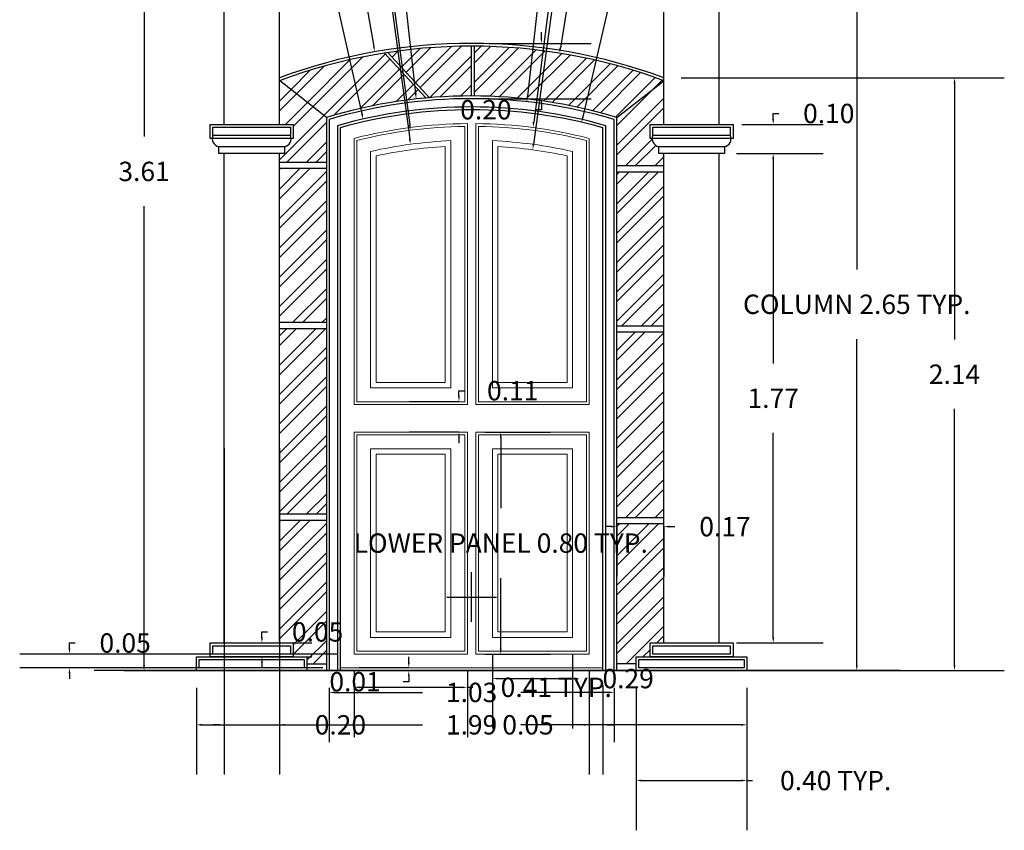
# Model space of a CAD drawing. Units: metres. Extents: x 10.71 to 14.27, y 9.22 to 13.79.
# Tile 1 of 2: x 10.71 to 14.27, y 9.22 to 12.15. Entities that reach past the tile are written whole.
import ezdxf

# ---------------------------------------------------------------- set-up
doc = ezdxf.new("R2010")
doc.units = ezdxf.units.M
doc.header["$MEASUREMENT"] = 0
for name, color, linetype, lineweight in [('A-ANNO-DIMS', 2, 'Continuous', 18), ('A-COLS', 7, 'Continuous', 30), ('A-DOOR', 4, 'Continuous', 18), ('A-DOOR-FRAM', 4, 'Continuous', 25), ('A-ELEV-GRND', 7, 'Continuous', 35), ('A-WALL', 7, 'Continuous', 25), ('A-WALL-PATT', 252, 'Continuous', 13)]:
    doc.layers.add(name, color=color, linetype=linetype, lineweight=lineweight)
doc.styles.get("Standard").update_dxf_attribs({"font": 'arial.ttf'})
doc.dimstyles.get("Standard").update_dxf_attribs({"dimtxt": 0.07, "dimasz": 0.02, "dimexe": 0.18, "dimexo": 0.0625, "dimgap": 0.09, "dimtad": 0, "dimtih": 1, "dimtoh": 1, "dimzin": 0, "dimdsep": 46, "dimtxsty": 'Standard', "dimcen": 0.09, "dimadec": 0, "dimazin": 0, "dimtfac": 1, "dimtofl": 0, "dimtmove": 0, "dimatfit": 3, "dimfxl": 1, "dimfxlon": 1, "dimtolj": 1, "dimtzin": 0, "dimarcsym": 0})

# ---------------------------------------------------------------- blocks, each defined once
blk = doc.blocks.new('*D1')
at = {"layer": 'A-ANNO-DIMS', "color": 0, "lineweight": -2, "transparency": 16777216}
for p, q in [((12.8472, 10.321), (12.8272, 10.321)), ((12.8672, 10.321), (12.8672, 10.141)), ((13.0372, 10.321), (13.0372, 10.141)), ((13.0572, 10.321), (13.0772, 10.321))]:
    blk.add_line(p, q, dxfattribs=at)
at = {"layer": 'A-ANNO-DIMS', "color": 0, "transparency": 16777216}
for points in [[(12.8472, 10.3244), (12.8472, 10.3177), (12.8672, 10.321)], [(13.0572, 10.3244), (13.0572, 10.3177), (13.0372, 10.321)]]:
    blk.add_solid(points, dxfattribs=at)
at = {"layer": 'Defpoints', "color": 0, "transparency": 16777216}
for p in [(12.8672, 10.332), (13.0372, 10.332), (13.0372, 10.321)]:
    blk.add_point(p, dxfattribs=at)
at = {"layer": 'A-ANNO-DIMS', "color": 0, "transparency": 16777216, "insert": (13.2581, 10.321), "char_height": 0.07, "attachment_point": 5}
blk.add_mtext('\\A1;0.17', dxfattribs=at)
blk = doc.blocks.new('*D2')
at = {"layer": 'A-ANNO-DIMS', "color": 0, "lineweight": -2, "transparency": 16777216}
for p, q in [((13.4325, 11.795), (13.4325, 11.815)), ((13.4325, 11.815), (13.4525, 11.815)), ((13.3185, 11.775), (13.6125, 11.775)), ((13.3185, 11.6703), (13.6125, 11.6703)), ((13.4325, 11.6503), (13.4325, 11.6303))]:
    blk.add_line(p, q, dxfattribs=at)
at = {"layer": 'A-ANNO-DIMS', "color": 0, "transparency": 16777216}
for points in [[(13.4291, 11.795), (13.4358, 11.795), (13.4325, 11.775)], [(13.4291, 11.6503), (13.4358, 11.6503), (13.4325, 11.6703)]]:
    blk.add_solid(points, dxfattribs=at)
at = {"layer": 'Defpoints', "color": 0, "transparency": 16777216}
for p in [(13.256, 11.775), (13.4325, 11.775), (13.256, 11.6703)]:
    blk.add_point(p, dxfattribs=at)
at = {"layer": 'A-ANNO-DIMS', "color": 0, "transparency": 16777216, "insert": (13.6333, 11.815), "char_height": 0.07, "attachment_point": 5}
blk.add_mtext('\\A1;0.10', dxfattribs=at)
blk = doc.blocks.new('*D3')
at = {"layer": 'A-ANNO-DIMS', "color": 0, "lineweight": -2, "transparency": 16777216}
for p, q in [((13.2997, 11.6703), (13.6125, 11.6703)), ((13.4325, 11.6503), (13.4325, 10.9104)), ((13.4325, 9.9203), (13.4325, 10.6601)), ((13.2997, 9.9003), (13.6125, 9.9003))]:
    blk.add_line(p, q, dxfattribs=at)
at = {"layer": 'A-ANNO-DIMS', "color": 0, "transparency": 16777216}
for points in [[(13.4291, 11.6503), (13.4358, 11.6503), (13.4325, 11.6703)], [(13.4291, 9.9203), (13.4358, 9.9203), (13.4325, 9.9003)]]:
    blk.add_solid(points, dxfattribs=at)
at = {"layer": 'Defpoints', "color": 0, "transparency": 16777216}
for p in [(13.2372, 11.6703), (13.4325, 11.6703), (13.2372, 9.9003)]:
    blk.add_point(p, dxfattribs=at)
at = {"layer": 'A-ANNO-DIMS', "color": 0, "transparency": 16777216, "insert": (13.4325, 10.7853), "char_height": 0.07, "attachment_point": 5}
blk.add_mtext('\\A1;1.77', dxfattribs=at)
blk = doc.blocks.new('*D4')
at = {"layer": 'A-ANNO-DIMS', "color": 0, "lineweight": -2, "transparency": 16777216}
for p, q in [((12.1582, 13.4108), (10.9782, 13.4108)), ((11.1582, 13.3908), (11.1582, 11.7313)), ((11.1582, 9.8203), (11.1582, 11.4798)), ((11.1582, 9.8003), (10.9782, 9.8003))]:
    blk.add_line(p, q, dxfattribs=at)
at = {"layer": 'A-ANNO-DIMS', "color": 0, "transparency": 16777216}
for points in [[(11.1548, 13.3908), (11.1615, 13.3908), (11.1582, 13.4108)], [(11.1548, 9.8203), (11.1615, 9.8203), (11.1582, 9.8003)]]:
    blk.add_solid(points, dxfattribs=at)
at = {"layer": 'Defpoints', "color": 0, "transparency": 16777216}
for p in [(11.1582, 13.4108), (12.3422, 13.4108), (11.1842, 9.8003)]:
    blk.add_point(p, dxfattribs=at)
at = {"layer": 'A-ANNO-DIMS', "color": 0, "transparency": 16777216, "insert": (11.1582, 11.6055), "char_height": 0.07, "attachment_point": 5}
blk.add_mtext('\\A1;3.61', dxfattribs=at)
blk = doc.blocks.new('*D6')
at = {"layer": 'A-ANNO-DIMS', "color": 0, "lineweight": -2, "transparency": 16777216}
for p, q in [((12.5946, 12.0885), (12.5946, 12.1085)), ((12.4047, 12.0685), (12.7746, 12.0685)), ((12.4047, 11.8685), (12.7746, 11.8685)), ((12.5946, 11.8285), (12.5746, 11.8285)), ((12.5946, 11.8485), (12.5946, 11.8285))]:
    blk.add_line(p, q, dxfattribs=at)
at = {"layer": 'A-ANNO-DIMS', "color": 0, "transparency": 16777216}
for points in [[(12.5912, 12.0885), (12.5979, 12.0885), (12.5946, 12.0685)], [(12.5912, 11.8485), (12.5979, 11.8485), (12.5946, 11.8685)]]:
    blk.add_solid(points, dxfattribs=at)
at = {"layer": 'Defpoints', "color": 0, "transparency": 16777216}
for p in [(12.3422, 12.0685), (12.3422, 11.8685), (12.5946, 11.8685)]:
    blk.add_point(p, dxfattribs=at)
at = {"layer": 'A-ANNO-DIMS', "color": 0, "transparency": 16777216, "insert": (12.3938, 11.8285), "char_height": 0.07, "attachment_point": 5}
blk.add_mtext('\\A1;0.20', dxfattribs=at)
blk = doc.blocks.new('*D7')
at = {"layer": 'A-ANNO-DIMS', "color": 0, "lineweight": -2, "transparency": 16777216}
for p, q in [((12.2966, 10.7926), (12.2966, 10.8126)), ((12.2966, 10.8126), (12.3166, 10.8126)), ((12.2966, 10.7726), (12.1166, 10.7726)), ((12.2966, 10.6626), (12.1166, 10.6626)), ((12.2966, 10.6426), (12.2966, 10.6226))]:
    blk.add_line(p, q, dxfattribs=at)
at = {"layer": 'A-ANNO-DIMS', "color": 0, "transparency": 16777216}
for points in [[(12.2933, 10.7926), (12.3, 10.7926), (12.2966, 10.7726)], [(12.2933, 10.6426), (12.3, 10.6426), (12.2966, 10.6626)]]:
    blk.add_solid(points, dxfattribs=at)
at = {"layer": 'Defpoints', "color": 0, "transparency": 16777216}
for p in [(12.2966, 10.7726), (12.3172, 10.7726), (12.3272, 10.6626)]:
    blk.add_point(p, dxfattribs=at)
at = {"layer": 'A-ANNO-DIMS', "color": 0, "transparency": 16777216, "insert": (12.4908, 10.8126), "char_height": 0.07, "attachment_point": 5}
blk.add_mtext('\\A1;0.11', dxfattribs=at)
blk = doc.blocks.new('*D8')
at = {"layer": 'A-ANNO-DIMS', "color": 0, "lineweight": -2, "transparency": 16777216}
for p, q in [((11.5843, 9.9203), (11.5843, 9.9403)), ((11.5843, 9.9403), (11.6043, 9.9403)), ((11.5843, 9.9003), (11.7643, 9.9003)), ((11.5843, 9.8503), (11.7643, 9.8503)), ((11.5843, 9.8303), (11.5843, 9.8103))]:
    blk.add_line(p, q, dxfattribs=at)
at = {"layer": 'A-ANNO-DIMS', "color": 0, "transparency": 16777216}
for points in [[(11.581, 9.9203), (11.5877, 9.9203), (11.5843, 9.9003)], [(11.581, 9.8303), (11.5877, 9.8303), (11.5843, 9.8503)]]:
    blk.add_solid(points, dxfattribs=at)
at = {"layer": 'Defpoints', "color": 0, "transparency": 16777216}
for p in [(11.5582, 9.9003), (11.5843, 9.9003), (11.5582, 9.8503)]:
    blk.add_point(p, dxfattribs=at)
at = {"layer": 'A-ANNO-DIMS', "color": 0, "transparency": 16777216, "insert": (11.7855, 9.9403), "char_height": 0.07, "attachment_point": 5}
blk.add_mtext('\\A1;0.05', dxfattribs=at)
blk = doc.blocks.new('*D10')
at = {"layer": 'A-ANNO-DIMS', "color": 0, "lineweight": -2, "transparency": 16777216}
for p, q in [((11.8272, 9.7378), (11.8272, 9.5415)), ((11.8472, 9.7215), (12.1646, 9.7215)), ((12.8372, 9.7215), (12.5198, 9.7215)), ((12.8572, 9.7378), (12.8572, 9.5415))]:
    blk.add_line(p, q, dxfattribs=at)
at = {"layer": 'A-ANNO-DIMS', "color": 0, "transparency": 16777216}
for points in [[(11.8472, 9.7248), (11.8472, 9.7182), (11.8272, 9.7215)], [(12.8372, 9.7248), (12.8372, 9.7182), (12.8572, 9.7215)]]:
    blk.add_solid(points, dxfattribs=at)
at = {"layer": 'Defpoints', "color": 0, "transparency": 16777216}
for p in [(11.8272, 9.8003), (12.8572, 9.8003), (12.8572, 9.7215)]:
    blk.add_point(p, dxfattribs=at)
at = {"layer": 'A-ANNO-DIMS', "color": 0, "transparency": 16777216, "insert": (12.3422, 9.7215), "char_height": 0.07, "attachment_point": 5}
blk.add_mtext('\\A1;1.03', dxfattribs=at)
blk = doc.blocks.new('*D11')
at = {"layer": 'A-ANNO-DIMS', "color": 0, "lineweight": -2, "transparency": 16777216}
for p, q in [((12.1152, 9.8302), (12.1152, 9.8502)), ((12.1152, 9.8102), (11.9352, 9.8102)), ((12.1152, 9.8003), (11.9352, 9.8003)), ((12.1152, 9.7603), (12.0952, 9.7603)), ((12.1152, 9.7803), (12.1152, 9.7603))]:
    blk.add_line(p, q, dxfattribs=at)
at = {"layer": 'A-ANNO-DIMS', "color": 0, "transparency": 16777216}
for points in [[(12.1118, 9.8302), (12.1185, 9.8302), (12.1152, 9.8102)], [(12.1118, 9.7803), (12.1185, 9.7803), (12.1152, 9.8003)]]:
    blk.add_solid(points, dxfattribs=at)
at = {"layer": 'Defpoints', "color": 0, "transparency": 16777216}
for p in [(12.1152, 9.8003), (12.1372, 9.8102), (12.1372, 9.8003)]:
    blk.add_point(p, dxfattribs=at)
at = {"layer": 'A-ANNO-DIMS', "color": 0, "transparency": 16777216, "insert": (11.921, 9.7603), "char_height": 0.07, "attachment_point": 5}
blk.add_mtext('\\A1;0.01', dxfattribs=at)
blk = doc.blocks.new('*D12')
at = {"layer": 'A-ANNO-DIMS', "color": 0, "lineweight": -2, "transparency": 16777216}
for p, q in [((12.4172, 9.8577), (12.4172, 9.5915)), ((12.7072, 9.8577), (12.7072, 9.5915)), ((12.4372, 9.7715), (12.6872, 9.7715)), ((12.7072, 9.7715), (12.7272, 9.7715))]:
    blk.add_line(p, q, dxfattribs=at)
at = {"layer": 'A-ANNO-DIMS', "color": 0, "transparency": 16777216}
for points in [[(12.4372, 9.7748), (12.4372, 9.7682), (12.4172, 9.7715)], [(12.6872, 9.7748), (12.6872, 9.7682), (12.7072, 9.7715)]]:
    blk.add_solid(points, dxfattribs=at)
at = {"layer": 'Defpoints', "color": 0, "transparency": 16777216}
for p in [(12.4172, 9.9202), (12.7072, 9.9202), (12.7072, 9.7715)]:
    blk.add_point(p, dxfattribs=at)
at = {"layer": 'A-ANNO-DIMS', "color": 0, "transparency": 16777216, "insert": (12.9082, 9.7715), "char_height": 0.07, "attachment_point": 5}
blk.add_mtext('\\A1;0.29', dxfattribs=at)
blk = doc.blocks.new('COL-ENTRANCE-CLASSICAL')
for p, q in [((0.1002, 1.975), (0.1002, 2.545)), ((0.3002, 1.975), (0.3002, 2.545)), ((0.1002, 0.1003), (0.1002, 1.8703)), ((0.3002, 0.1003), (0.3002, 1.8703)), ((0.1002, 0.1003), (0.3002, 0.1003))]:
    blk.add_line(p, q)
for points in [[(0.0502, 2.6498), (0.3502, 2.6498), (0.3502, 2.5998), (0.0502, 2.5998)], [(0.0602, 2.6398), (0.3402, 2.6398), (0.3402, 2.6098), (0.0602, 2.6098)], [(0.0816, 2.5705), (0.319, 2.5705), (0.319, 2.545), (0.0816, 2.545)], [(0.0502, 1.975), (0.3502, 1.975), (0.3502, 1.925), (0.0502, 1.925)], [(0.0602, 1.965), (0.3402, 1.965), (0.3402, 1.935), (0.0602, 1.935)], [(0.0816, 1.8957), (0.319, 1.8957), (0.319, 1.8703), (0.0816, 1.8703)], [(0.0502, 0.1003), (0.3502, 0.1003), (0.3502, 0.0503), (0.0502, 0.0503)], [(0.0602, 0.0903), (0.3402, 0.0903), (0.3402, 0.0603), (0.0602, 0.0603)], [(0.0002, 0.0503), (0.4002, 0.0503), (0.4002, 0.0003), (0.0002, 0.0003)], [(0.0102, 0.0403), (0.3902, 0.0403), (0.3902, 0.0103), (0.0102, 0.0103)]]:
    blk.add_lwpolyline(points, close=True)
for centre, radius, start, end in [((0.0856, 2.5981), 0.0279, 155.2605, 261.7776), ((0.3152, 2.5979), 0.0277, 277.9826, 25.4449), ((0.0856, 1.9233), 0.0279, 155.2605, 261.7776), ((0.3152, 1.9231), 0.0277, 277.9826, 25.4449)]:
    blk.add_arc(centre, radius, start, end)
blk = doc.blocks.new('DOOR-PANEL-LOWER')
for points in [[(0.4102, 0.8026), (0.4102, 0.0002), (0.0002, 0.0002), (0.0002, 0.8026)], [(0.4002, 0.7926), (0.4002, 0.0102), (0.0102, 0.0102), (0.0102, 0.7926)], [(0.3502, 0.7426), (0.3502, 0.0602), (0.0602, 0.0602), (0.0602, 0.7426)], [(0.3302, 0.7226), (0.3302, 0.0802), (0.0802, 0.0802), (0.0802, 0.7226)]]:
    blk.add_lwpolyline(points, close=True)
blk = doc.blocks.new('*D15')
at = {"layer": 'A-ANNO-DIMS', "color": 0, "lineweight": -2, "transparency": 16777216}
for p, q in [((13.3997, 12.4498), (13.9146, 12.4498)), ((13.7346, 12.4298), (13.7346, 11.2512)), ((13.7346, 9.8203), (13.7346, 10.9988)), ((13.3997, 9.8003), (13.9146, 9.8003))]:
    blk.add_line(p, q, dxfattribs=at)
at = {"layer": 'A-ANNO-DIMS', "color": 0, "transparency": 16777216}
for points in [[(13.7313, 12.4298), (13.738, 12.4298), (13.7346, 12.4498)], [(13.7313, 9.8203), (13.738, 9.8203), (13.7346, 9.8003)]]:
    blk.add_solid(points, dxfattribs=at)
at = {"layer": 'Defpoints', "color": 0, "transparency": 16777216}
for p in [(13.3372, 12.4498), (13.7346, 12.4498), (13.3372, 9.8003)]:
    blk.add_point(p, dxfattribs=at)
at = {"layer": 'A-ANNO-DIMS', "color": 0, "transparency": 16777216, "insert": (13.7346, 11.125), "char_height": 0.07, "attachment_point": 5}
blk.add_mtext('\\A1;COLUMN 2.65 TYP.', dxfattribs=at)
blk = doc.blocks.new('*D16')
at = {"layer": 'A-ANNO-DIMS', "color": 0, "lineweight": -2, "transparency": 16777216}
for p, q in [((12.9372, 9.7378), (12.9372, 9.2228)), ((13.3372, 9.7378), (13.3372, 9.2228)), ((12.9572, 9.4028), (13.3172, 9.4028)), ((13.3372, 9.4028), (13.3572, 9.4028))]:
    blk.add_line(p, q, dxfattribs=at)
at = {"layer": 'A-ANNO-DIMS', "color": 0, "transparency": 16777216}
for points in [[(12.9572, 9.4062), (12.9572, 9.3995), (12.9372, 9.4028)], [(13.3172, 9.4062), (13.3172, 9.3995), (13.3372, 9.4028)]]:
    blk.add_solid(points, dxfattribs=at)
at = {"layer": 'Defpoints', "color": 0, "transparency": 16777216}
for p in [(12.9372, 9.8003), (13.3372, 9.8003), (13.3372, 9.4028)]:
    blk.add_point(p, dxfattribs=at)
at = {"layer": 'A-ANNO-DIMS', "color": 0, "transparency": 16777216, "insert": (13.6583, 9.4028), "char_height": 0.07, "attachment_point": 5}
blk.add_mtext('\\A1;0.40 TYP.', dxfattribs=at)
blk = doc.blocks.new('*D17')
at = {"layer": 'A-ANNO-DIMS', "color": 0, "lineweight": -2, "transparency": 16777216}
for p, q in [((12.3897, 10.6626), (12.6276, 10.6626)), ((12.4476, 10.6426), (12.4476, 10.3876)), ((12.4476, 9.8802), (12.4476, 10.1352)), ((12.3897, 9.8602), (12.6276, 9.8602))]:
    blk.add_line(p, q, dxfattribs=at)
at = {"layer": 'A-ANNO-DIMS', "color": 0, "transparency": 16777216}
for points in [[(12.4442, 10.6426), (12.4509, 10.6426), (12.4476, 10.6626)], [(12.4442, 9.8802), (12.4509, 9.8802), (12.4476, 9.8602)]]:
    blk.add_solid(points, dxfattribs=at)
at = {"layer": 'Defpoints', "color": 0, "transparency": 16777216}
for p in [(12.3272, 10.6626), (12.4476, 10.6626), (12.3272, 9.8602)]:
    blk.add_point(p, dxfattribs=at)
at = {"layer": 'A-ANNO-DIMS', "color": 0, "transparency": 16777216, "insert": (12.4476, 10.2614), "char_height": 0.07, "attachment_point": 5}
blk.add_mtext('\\A1;LOWER PANEL 0.80 TYP.', dxfattribs=at)
blk = doc.blocks.new('*D18')
at = {"layer": 'A-ANNO-DIMS', "color": 0, "lineweight": -2, "transparency": 16777216}
for p, q in [((11.9172, 9.7977), (11.9172, 9.5599)), ((12.3272, 9.7977), (12.3272, 9.5599)), ((11.9372, 9.7399), (12.3072, 9.7399)), ((12.3272, 9.7399), (12.3472, 9.7399))]:
    blk.add_line(p, q, dxfattribs=at)
at = {"layer": 'A-ANNO-DIMS', "color": 0, "transparency": 16777216}
for points in [[(11.9372, 9.7432), (11.9372, 9.7365), (11.9172, 9.7399)], [(12.3072, 9.7432), (12.3072, 9.7365), (12.3272, 9.7399)]]:
    blk.add_solid(points, dxfattribs=at)
at = {"layer": 'Defpoints', "color": 0, "transparency": 16777216}
for p in [(11.9172, 9.8602), (12.3272, 9.8602), (12.3272, 9.7399)]:
    blk.add_point(p, dxfattribs=at)
at = {"layer": 'A-ANNO-DIMS', "color": 0, "transparency": 16777216, "insert": (12.6483, 9.7399), "char_height": 0.07, "attachment_point": 5}
blk.add_mtext('\\A1;0.41 TYP.', dxfattribs=at)
blk = doc.blocks.new('*D22')
at = {"layer": 'A-ANNO-DIMS', "color": 0, "lineweight": -2, "transparency": 16777216}
for p, q in [((11.3472, 9.7378), (11.3472, 9.4243)), ((13.3372, 9.7378), (13.3372, 9.4243)), ((11.3672, 9.6043), (12.1645, 9.6043)), ((13.3172, 9.6043), (12.5199, 9.6043))]:
    blk.add_line(p, q, dxfattribs=at)
at = {"layer": 'A-ANNO-DIMS', "color": 0, "transparency": 16777216}
for points in [[(11.3672, 9.6076), (11.3672, 9.6009), (11.3472, 9.6043)], [(13.3172, 9.6076), (13.3172, 9.6009), (13.3372, 9.6043)]]:
    blk.add_solid(points, dxfattribs=at)
at = {"layer": 'Defpoints', "color": 0, "transparency": 16777216}
for p in [(11.3472, 9.8003), (13.3372, 9.8003), (13.3372, 9.6043)]:
    blk.add_point(p, dxfattribs=at)
at = {"layer": 'A-ANNO-DIMS', "color": 0, "transparency": 16777216, "insert": (12.3422, 9.6043), "char_height": 0.07, "attachment_point": 5}
blk.add_mtext('\\A1;1.99', dxfattribs=at)
blk = doc.blocks.new('*D23')
at = {"layer": 'A-ANNO-DIMS', "color": 0, "lineweight": -2, "transparency": 16777216}
for p, q in [((13.0997, 11.944), (14.2679, 11.944)), ((14.0879, 11.924), (14.0879, 10.9973)), ((14.0879, 9.8203), (14.0879, 10.747)), ((13.3997, 9.8003), (14.2679, 9.8003))]:
    blk.add_line(p, q, dxfattribs=at)
at = {"layer": 'A-ANNO-DIMS', "color": 0, "transparency": 16777216}
for points in [[(14.0846, 11.924), (14.0912, 11.924), (14.0879, 11.944)], [(14.0846, 9.8203), (14.0912, 9.8203), (14.0879, 9.8003)]]:
    blk.add_solid(points, dxfattribs=at)
at = {"layer": 'Defpoints', "color": 0, "transparency": 16777216}
for p in [(13.0372, 11.944), (14.0879, 11.944), (13.3372, 9.8003)]:
    blk.add_point(p, dxfattribs=at)
at = {"layer": 'A-ANNO-DIMS', "color": 0, "transparency": 16777216, "insert": (14.0879, 10.8721), "char_height": 0.07, "attachment_point": 5}
blk.add_mtext('\\A1;2.14', dxfattribs=at)
blk = doc.blocks.new('*D24')
at = {"layer": 'A-ANNO-DIMS', "color": 0, "lineweight": -2, "transparency": 16777216}
for p, q in [((11.3972, 12.6068), (11.3972, 13.7868)), ((11.6972, 12.6068), (11.6972, 13.7868)), ((11.4172, 13.6068), (11.6772, 13.6068)), ((11.6972, 13.6068), (11.7172, 13.6068))]:
    blk.add_line(p, q, dxfattribs=at)
at = {"layer": 'A-ANNO-DIMS', "color": 0, "transparency": 16777216}
for points in [[(11.4172, 13.6101), (11.4172, 13.6035), (11.3972, 13.6068)], [(11.6772, 13.6101), (11.6772, 13.6035), (11.6972, 13.6068)]]:
    blk.add_solid(points, dxfattribs=at)
at = {"layer": 'Defpoints', "color": 0, "transparency": 16777216}
for p in [(11.6972, 13.6068), (11.3972, 11.775), (11.6972, 11.775)]:
    blk.add_point(p, dxfattribs=at)
at = {"layer": 'A-ANNO-DIMS', "color": 0, "transparency": 16777216, "insert": (11.898, 13.6068), "char_height": 0.07, "attachment_point": 5}
blk.add_mtext('\\A1;0.30', dxfattribs=at)
blk = doc.blocks.new('*D25')
at = {"layer": 'A-ANNO-DIMS', "color": 0, "lineweight": -2, "transparency": 16777216}
for p, q in [((11.4472, 10.6043), (11.4472, 9.4243)), ((11.6472, 10.6043), (11.6472, 9.4243)), ((11.4272, 9.6043), (11.4072, 9.6043)), ((11.6672, 9.6043), (11.6872, 9.6043))]:
    blk.add_line(p, q, dxfattribs=at)
at = {"layer": 'A-ANNO-DIMS', "color": 0, "transparency": 16777216}
for points in [[(11.4272, 9.6076), (11.4272, 9.6009), (11.4472, 9.6043)], [(11.6672, 9.6076), (11.6672, 9.6009), (11.6472, 9.6043)]]:
    blk.add_solid(points, dxfattribs=at)
at = {"layer": 'Defpoints', "color": 0, "transparency": 16777216}
for p in [(11.4472, 11.6703), (11.6472, 11.6703), (11.6472, 9.6043)]:
    blk.add_point(p, dxfattribs=at)
at = {"layer": 'A-ANNO-DIMS', "color": 0, "transparency": 16777216, "insert": (11.868, 9.6043), "char_height": 0.07, "attachment_point": 5}
blk.add_mtext('\\A1;0.20', dxfattribs=at)
blk = doc.blocks.new('*D26')
at = {"layer": 'A-ANNO-DIMS', "color": 0, "lineweight": -2, "transparency": 16777216}
for p, q in [((10.8886, 9.8802), (10.8886, 9.9002)), ((10.8886, 9.9002), (10.9086, 9.9002)), ((11.8547, 9.8602), (10.7086, 9.8602)), ((11.8047, 9.8102), (10.7086, 9.8102)), ((10.8886, 9.7902), (10.8886, 9.7702))]:
    blk.add_line(p, q, dxfattribs=at)
at = {"layer": 'A-ANNO-DIMS', "color": 0, "transparency": 16777216}
for points in [[(10.8853, 9.8802), (10.892, 9.8802), (10.8886, 9.8602)], [(10.8853, 9.7902), (10.892, 9.7902), (10.8886, 9.8102)]]:
    blk.add_solid(points, dxfattribs=at)
at = {"layer": 'Defpoints', "color": 0, "transparency": 16777216}
for p in [(10.8886, 9.8602), (11.9172, 9.8602), (11.8672, 9.8102)]:
    blk.add_point(p, dxfattribs=at)
at = {"layer": 'A-ANNO-DIMS', "color": 0, "transparency": 16777216, "insert": (11.0898, 9.9002), "char_height": 0.07, "attachment_point": 5}
blk.add_mtext('\\A1;0.05', dxfattribs=at)
blk = doc.blocks.new('*D27')
at = {"layer": 'A-ANNO-DIMS', "color": 0, "lineweight": -2, "transparency": 16777216}
for p, q in [((12.7672, 9.7977), (12.7672, 9.4243)), ((12.8172, 9.7477), (12.8172, 9.4243)), ((12.7472, 9.6043), (12.7272, 9.6043)), ((12.8372, 9.6043), (12.8572, 9.6043))]:
    blk.add_line(p, q, dxfattribs=at)
at = {"layer": 'A-ANNO-DIMS', "color": 0, "transparency": 16777216}
for points in [[(12.7472, 9.6076), (12.7472, 9.6009), (12.7672, 9.6043)], [(12.8372, 9.6076), (12.8372, 9.6009), (12.8172, 9.6043)]]:
    blk.add_solid(points, dxfattribs=at)
at = {"layer": 'Defpoints', "color": 0, "transparency": 16777216}
for p in [(12.7672, 9.8602), (12.8172, 9.8102), (12.7672, 9.6043)]:
    blk.add_point(p, dxfattribs=at)
at = {"layer": 'A-ANNO-DIMS', "color": 0, "transparency": 16777216, "insert": (12.546, 9.6043), "char_height": 0.07, "attachment_point": 5}
blk.add_mtext('\\A1;0.05', dxfattribs=at)
blk = doc.blocks.new('*D28')
at = {"layer": 'A-ANNO-DIMS', "color": 0, "lineweight": -2, "transparency": 16777216}
for p, q in [((11.762, 13.2204), (11.782, 13.2204)), ((11.782, 13.2204), (11.9886, 12.0574)), ((12.3422, 9.9765), (12.3422, 10.1565)), ((12.2522, 10.0665), (12.4322, 10.0665))]:
    blk.add_line(p, q, dxfattribs=at)
at = {"layer": 'A-ANNO-DIMS', "color": 0, "transparency": 16777216}
blk.add_solid([(11.9918, 12.058), (11.9853, 12.0568), (11.9921, 12.0377)], dxfattribs=at)
at = {"layer": 'Defpoints', "color": 0, "transparency": 16777216}
for p in [(11.9921, 12.0377), (12.3422, 10.0665)]:
    blk.add_point(p, dxfattribs=at)
at = {"layer": 'A-ANNO-DIMS', "color": 0, "transparency": 16777216, "insert": (11.5207, 13.2204), "char_height": 0.07, "attachment_point": 5}
blk.add_mtext('\\A1;R2.002', dxfattribs=at)
blk = doc.blocks.new('*D29')
at = {"layer": 'A-ANNO-DIMS', "color": 0, "lineweight": -2, "transparency": 16777216}
for p, q in [((12.8507, 13.2129), (12.6632, 12.0528)), ((12.8707, 13.2129), (12.8507, 13.2129)), ((12.3422, 9.9765), (12.3422, 10.1565)), ((12.2522, 10.0665), (12.4322, 10.0665))]:
    blk.add_line(p, q, dxfattribs=at)
at = {"layer": 'A-ANNO-DIMS', "color": 0, "transparency": 16777216}
blk.add_solid([(12.6599, 12.0533), (12.6665, 12.0522), (12.66, 12.033)], dxfattribs=at)
at = {"layer": 'Defpoints', "color": 0, "transparency": 16777216}
for p in [(12.66, 12.033), (12.3422, 10.0665)]:
    blk.add_point(p, dxfattribs=at)
at = {"layer": 'A-ANNO-DIMS', "color": 0, "transparency": 16777216, "insert": (13.1119, 13.2129), "char_height": 0.07, "attachment_point": 5}
blk.add_mtext('\\A1;R1.992', dxfattribs=at)
blk = doc.blocks.new('*D30')
at = {"layer": 'A-ANNO-DIMS', "color": 0, "lineweight": -2, "transparency": 16777216}
for p, q in [((12.002, 12.948), (12.022, 12.948)), ((12.022, 12.948), (12.1399, 11.8873)), ((12.3422, 9.9765), (12.3422, 10.1565)), ((12.2522, 10.0665), (12.4322, 10.0665))]:
    blk.add_line(p, q, dxfattribs=at)
at = {"layer": 'A-ANNO-DIMS', "color": 0, "transparency": 16777216}
blk.add_solid([(12.1432, 11.8877), (12.1365, 11.887), (12.1421, 11.8675)], dxfattribs=at)
at = {"layer": 'Defpoints', "color": 0, "transparency": 16777216}
for p in [(12.1421, 11.8675), (12.3422, 10.0665)]:
    blk.add_point(p, dxfattribs=at)
at = {"layer": 'A-ANNO-DIMS', "color": 0, "transparency": 16777216, "insert": (11.7607, 12.948), "char_height": 0.07, "attachment_point": 5}
blk.add_mtext('\\A1;R1.812', dxfattribs=at)
blk = doc.blocks.new('*D31')
at = {"layer": 'A-ANNO-DIMS', "color": 0, "lineweight": -2, "transparency": 16777216}
for p, q in [((12.6618, 12.932), (12.5442, 11.8773)), ((12.6818, 12.932), (12.6618, 12.932)), ((12.3422, 9.9765), (12.3422, 10.1565)), ((12.2522, 10.0665), (12.4322, 10.0665))]:
    blk.add_line(p, q, dxfattribs=at)
at = {"layer": 'A-ANNO-DIMS', "color": 0, "transparency": 16777216}
blk.add_solid([(12.5408, 11.8777), (12.5475, 11.8769), (12.5419, 11.8574)], dxfattribs=at)
at = {"layer": 'Defpoints', "color": 0, "transparency": 16777216}
for p in [(12.5419, 11.8574), (12.3422, 10.0665)]:
    blk.add_point(p, dxfattribs=at)
at = {"layer": 'A-ANNO-DIMS', "color": 0, "transparency": 16777216, "insert": (12.923, 12.932), "char_height": 0.07, "attachment_point": 5}
blk.add_mtext('\\A1;R1.802', dxfattribs=at)
blk = doc.blocks.new('*D32')
at = {"layer": 'A-ANNO-DIMS', "color": 0, "lineweight": -2, "transparency": 16777216}
for p, q in [((11.6948, 12.8315), (11.7148, 12.8315)), ((11.7148, 12.8315), (11.9457, 11.8141)), ((12.3422, 9.9765), (12.3422, 10.1565)), ((12.2522, 10.0665), (12.4322, 10.0665))]:
    blk.add_line(p, q, dxfattribs=at)
at = {"layer": 'A-ANNO-DIMS', "color": 0, "transparency": 16777216}
blk.add_solid([(11.9489, 11.8149), (11.9424, 11.8134), (11.9501, 11.7946)], dxfattribs=at)
at = {"layer": 'Defpoints', "color": 0, "transparency": 16777216}
for p in [(11.9501, 11.7946), (12.3422, 10.0665)]:
    blk.add_point(p, dxfattribs=at)
at = {"layer": 'A-ANNO-DIMS', "color": 0, "transparency": 16777216, "insert": (11.4536, 12.8315), "char_height": 0.07, "attachment_point": 5}
blk.add_mtext('\\A1;R1.772', dxfattribs=at)
blk = doc.blocks.new('*D33')
at = {"layer": 'A-ANNO-DIMS', "color": 0, "lineweight": -2, "transparency": 16777216}
for p, q in [((12.9783, 12.8131), (12.7443, 11.8026)), ((12.9983, 12.8131), (12.9783, 12.8131)), ((12.3422, 9.9765), (12.3422, 10.1565)), ((12.2522, 10.0665), (12.4322, 10.0665))]:
    blk.add_line(p, q, dxfattribs=at)
at = {"layer": 'A-ANNO-DIMS', "color": 0, "transparency": 16777216}
blk.add_solid([(12.7411, 11.8033), (12.7476, 11.8018), (12.7398, 11.7831)], dxfattribs=at)
at = {"layer": 'Defpoints', "color": 0, "transparency": 16777216}
for p in [(12.7398, 11.7831), (12.3422, 10.0665)]:
    blk.add_point(p, dxfattribs=at)
at = {"layer": 'A-ANNO-DIMS', "color": 0, "transparency": 16777216, "insert": (13.2396, 12.8131), "char_height": 0.07, "attachment_point": 5}
blk.add_mtext('\\A1;R1.762', dxfattribs=at)
blk = doc.blocks.new('*D34')
at = {"layer": 'A-ANNO-DIMS', "color": 0, "lineweight": -2, "transparency": 16777216}
for p, q in [((12.6971, 12.7827), (12.5666, 11.7839)), ((12.7171, 12.7827), (12.6971, 12.7827)), ((12.3422, 9.9765), (12.3422, 10.1565)), ((12.2522, 10.0665), (12.4322, 10.0665))]:
    blk.add_line(p, q, dxfattribs=at)
at = {"layer": 'A-ANNO-DIMS', "color": 0, "transparency": 16777216}
blk.add_solid([(12.5633, 11.7844), (12.5699, 11.7835), (12.564, 11.7641)], dxfattribs=at)
at = {"layer": 'Defpoints', "color": 0, "transparency": 16777216}
for p in [(12.564, 11.7641), (12.3422, 10.0665)]:
    blk.add_point(p, dxfattribs=at)
at = {"layer": 'A-ANNO-DIMS', "color": 0, "transparency": 16777216, "insert": (13.0341, 12.7827), "char_height": 0.07, "attachment_point": 5}
blk.add_mtext('\\A1;2X R1.712', dxfattribs=at)
blk = doc.blocks.new('*D35')
at = {"layer": 'A-ANNO-DIMS', "color": 0, "lineweight": -2, "transparency": 16777216}
for p, q in [((11.9683, 12.7667), (11.9883, 12.7667)), ((11.9883, 12.7667), (12.1184, 11.7739)), ((12.3422, 9.9765), (12.3422, 10.1565)), ((12.2522, 10.0665), (12.4322, 10.0665))]:
    blk.add_line(p, q, dxfattribs=at)
at = {"layer": 'A-ANNO-DIMS', "color": 0, "transparency": 16777216}
blk.add_solid([(12.1217, 11.7744), (12.1151, 11.7735), (12.121, 11.7541)], dxfattribs=at)
at = {"layer": 'Defpoints', "color": 0, "transparency": 16777216}
for p in [(12.121, 11.7541), (12.3422, 10.0665)]:
    blk.add_point(p, dxfattribs=at)
at = {"layer": 'A-ANNO-DIMS', "color": 0, "transparency": 16777216, "insert": (11.6512, 12.7667), "char_height": 0.07, "attachment_point": 5}
blk.add_mtext('\\A1;2X R1.702', dxfattribs=at)
blk = doc.blocks.new('*D36')
at = {"layer": 'A-ANNO-DIMS', "color": 0, "lineweight": -2, "transparency": 16777216}
for p, q in [((11.9683, 12.686), (11.9883, 12.686)), ((11.9883, 12.686), (12.1184, 11.7235)), ((12.3422, 9.9765), (12.3422, 10.1565)), ((12.2522, 10.0665), (12.4322, 10.0665))]:
    blk.add_line(p, q, dxfattribs=at)
at = {"layer": 'A-ANNO-DIMS', "color": 0, "transparency": 16777216}
blk.add_solid([(12.1217, 11.7239), (12.1151, 11.723), (12.121, 11.7037)], dxfattribs=at)
at = {"layer": 'Defpoints', "color": 0, "transparency": 16777216}
for p in [(12.121, 11.7037), (12.3422, 10.0665)]:
    blk.add_point(p, dxfattribs=at)
at = {"layer": 'A-ANNO-DIMS', "color": 0, "transparency": 16777216, "insert": (11.6513, 12.686), "char_height": 0.07, "attachment_point": 5}
blk.add_mtext('\\A1;2X R1.652', dxfattribs=at)
blk = doc.blocks.new('*D37')
at = {"layer": 'A-ANNO-DIMS', "color": 0, "lineweight": -2, "transparency": 16777216}
for p, q in [((12.6954, 12.6538), (12.5656, 11.7034)), ((12.7154, 12.6538), (12.6954, 12.6538)), ((12.3422, 9.9765), (12.3422, 10.1565)), ((12.2522, 10.0665), (12.4322, 10.0665))]:
    blk.add_line(p, q, dxfattribs=at)
at = {"layer": 'A-ANNO-DIMS', "color": 0, "transparency": 16777216}
blk.add_solid([(12.5623, 11.7038), (12.5689, 11.7029), (12.5629, 11.6835)], dxfattribs=at)
at = {"layer": 'Defpoints', "color": 0, "transparency": 16777216}
for p in [(12.5629, 11.6835), (12.3422, 10.0665)]:
    blk.add_point(p, dxfattribs=at)
at = {"layer": 'A-ANNO-DIMS', "color": 0, "transparency": 16777216, "insert": (13.0324, 12.6538), "char_height": 0.07, "attachment_point": 5}
blk.add_mtext('\\A1;2X R1.632', dxfattribs=at)

msp = doc.modelspace()

# ---------------------------------------------------------------- hatches: boundary and pattern name
at = {"layer": 'A-WALL-PATT'}
h = msp.add_hatch(dxfattribs=at)
h.set_pattern_fill('ANSI32', color=256, scale=0.2)
h.paths.add_polyline_path([(12.9947, 11.725), (12.9872, 11.725), (12.9872, 11.775), (13.0372, 11.775), (13.0372, 11.9335), (12.8672, 11.8008), (12.8672, 11.6265), (13.0372, 11.6265), (13.0372, 11.6703), (13.0186, 11.6703), (13.0186, 11.6957, -0.390051)])
h.paths.add_polyline_path([(13.0372, 11.6042), (12.8672, 11.6042), (12.8672, 11.0473), (13.0372, 11.0473)])
h.paths.add_polyline_path([(12.3522, 12.0585), (12.3522, 11.8785, -0.072231), (12.8672, 11.8008), (13.0371, 11.9334, 0.088055)])
h.paths.add_polyline_path([(12.3422, 12.0585, 0.038132), (12.0397, 12.0354), (12.1896, 11.8721, -0.02108), (12.3422, 11.8785)])
h.paths.add_polyline_path([(12.0278, 12.0336, 0.049471), (11.6475, 11.9335), (11.8172, 11.8008, -0.050713), (12.1771, 11.871)])
h.paths.add_polyline_path([(11.8172, 11.8008), (11.6472, 11.9337), (11.6472, 11.775), (11.6972, 11.775), (11.6972, 11.725), (11.6898, 11.725, -0.393617), (11.666, 11.6957), (11.666, 11.6703), (11.6472, 11.6703), (11.6472, 11.639), (11.8172, 11.639)])
h.paths.add_polyline_path([(11.8172, 11.6167), (11.6472, 11.6167), (11.6472, 11.0598), (11.8172, 11.0598)])
h.paths.add_polyline_path([(11.8172, 11.0375), (11.6472, 11.0375), (11.6472, 10.3669), (11.8172, 10.3669)])
h.paths.add_polyline_path([(11.8172, 10.3445), (11.6472, 10.3445), (11.6472, 9.9003), (11.6972, 9.9003), (11.6972, 9.8503), (11.7472, 9.8503), (11.7472, 9.8253), (11.8172, 9.8253)])
h.paths.add_polyline_path([(13.0372, 10.332), (12.8672, 10.332), (12.8672, 9.8253), (12.9372, 9.8253), (12.9372, 9.8503), (12.9872, 9.8503), (12.9872, 9.9003), (13.0372, 9.9003)])
h.paths.add_polyline_path([(13.0372, 11.0249), (12.8672, 11.0249), (12.8672, 10.3543), (13.0372, 10.3543)])

# ---------------------------------------------------------------- linework, layer by layer
at = {"layer": 'A-DOOR'}
for p, q in [((12.3172, 11.7784), (12.3172, 11.7785)), ((12.3572, 11.7785), (12.3572, 11.7785)), ((12.3672, 11.7784), (12.3672, 11.7785)), ((11.8672, 9.8102), (12.3172, 9.8102)), ((12.3172, 9.8102), (12.8172, 9.8102)), ((12.628, 9.8102), (12.628, 9.8102))]:
    msp.add_line(p, q, dxfattribs=at)
msp.add_lwpolyline([(12.3272, 11.7785, 0.0606), (11.9172, 11.725), (11.9172, 10.7626), (12.3272, 10.7626), (12.3272, 11.7785)], format="xyb", dxfattribs=at)
for points in [[(12.3172, 10.7726), (12.3172, 11.7684, 0.05797), (11.9272, 11.7172), (11.9272, 10.7726)], [(12.7672, 10.7626), (12.7672, 11.725, 0.0606), (12.3572, 11.7785), (12.3572, 10.7626)], [(12.7572, 10.7726), (12.7572, 11.7172, 0.05797), (12.3672, 11.7684), (12.3672, 10.7726)], [(12.2672, 10.8226), (12.2672, 11.7168, 0.04437), (11.9772, 11.6777), (11.9772, 10.8226)], [(12.7072, 10.8226), (12.7072, 11.6777, 0.04437), (12.4172, 11.7168), (12.4172, 10.8226)], [(12.2472, 10.8426), (12.2472, 11.6958, 0.038708), (11.9972, 11.6617), (11.9972, 10.8426)], [(12.6872, 10.8426), (12.6872, 11.6617, 0.038708), (12.4372, 11.6958), (12.4372, 10.8426)]]:
    msp.add_lwpolyline(points, format="xyb", close=True, dxfattribs=at)
at = {"layer": 'A-DOOR-FRAM'}
for points in [[(12.8672, 9.8003), (12.8672, 11.8008, 0.148039), (11.8172, 11.8008), (11.8172, 9.8003)], [(12.8572, 9.8003), (12.8572, 11.7934, 0.145937), (11.8272, 11.7934), (11.8272, 9.8003)], [(12.8272, 9.8003), (12.8272, 11.7709, 0.139511), (11.8572, 11.7709), (11.8572, 9.8003)], [(12.8172, 9.8003), (12.8172, 11.7633, 0.137329), (11.8672, 11.7633), (11.8672, 9.8003)]]:
    msp.add_lwpolyline(points, format="xyb", dxfattribs=at)
at = {"layer": 'A-ELEV-GRND'}
for p, q in [((11.0846, 9.8003), (12.3272, 9.8003)), ((12.3272, 9.8003), (13.8919, 9.8003))]:
    msp.add_line(p, q, dxfattribs=at)
at = {"layer": 'A-WALL'}
for p, q in [((12.1771, 11.871), (12.0278, 12.0336)), ((12.1896, 11.8721), (12.0397, 12.0354)), ((12.3422, 11.8785), (12.3422, 12.0585)), ((12.3522, 11.8785), (12.3522, 12.0585)), ((11.8172, 11.8008), (11.6472, 11.9337)), ((12.8672, 11.8008), (13.0372, 11.9335)), ((11.6472, 11.639), (11.8172, 11.639)), ((11.6472, 11.6167), (11.8172, 11.6167)), ((12.8672, 11.6265), (13.0372, 11.6265)), ((12.8672, 11.6042), (13.0372, 11.6042)), ((11.6472, 11.0598), (11.8172, 11.0598)), ((11.6472, 11.0375), (11.8172, 11.0375)), ((12.8672, 11.0473), (13.0372, 11.0473)), ((12.8672, 11.0249), (13.0372, 11.0249)), ((11.6472, 10.3669), (11.8172, 10.3669)), ((11.6472, 10.3445), (11.8172, 10.3445)), ((12.8672, 10.3543), (13.0372, 10.3543)), ((12.8672, 10.332), (13.0372, 10.332)), ((11.7472, 9.8253), (11.8172, 9.8253)), ((12.9372, 9.8253), (12.8672, 9.8253))]:
    msp.add_line(p, q, dxfattribs=at)
for radius, start, end in [(2.002, 69.6872, 110.3128), (1.992, 69.5836, 110.4093)]:
    msp.add_arc((12.3422, 10.0665), radius, start, end, dxfattribs=at)

# ---------------------------------------------------------------- block references
at = {"layer": 'A-COLS'}
for p in [(11.347, 9.8), (12.937, 9.8)]:
    msp.add_blockref('COL-ENTRANCE-CLASSICAL', p, dxfattribs=at)
at = {"layer": 'A-DOOR'}
msp.add_blockref('DOOR-PANEL-LOWER', (11.917, 9.86), dxfattribs=at)
at = {"layer": 'A-DOOR', "extrusion": (0, 0, -1), "zscale": -1, "rotation": 180}
msp.add_blockref('DOOR-PANEL-LOWER', (-12.357, 10.6628), dxfattribs=at)

# ---------------------------------------------------------------- dimensions: what is measured, and where the dimension line sits
at = {"layer": 'A-ANNO-DIMS'}
for base, p1, p2, override, picture, middle in [((11.6972, 13.6068), (11.3972, 11.775), (11.6972, 11.775), {"dimdec": 2, "dimlfac": 1, "dimrnd": 0, "dimzin": 0, "dimdsep": 46, "dimlunit": 2}, '*D24', (11.898, 13.6068)), ((11.6472, 9.6043), (11.4472, 11.6703), (11.6472, 11.6703), {"dimdec": 2, "dimlfac": 1, "dimrnd": 0, "dimzin": 0, "dimdsep": 46, "dimlunit": 2}, '*D25', (11.868, 9.6043)), ((13.0372, 10.321), (12.8672, 10.332), (13.0372, 10.332), {"dimclrd": 0, "dimclre": 0, "dimclrt": 0}, '*D1', (13.2581, 10.321)), ((12.7072, 9.7715), (12.4172, 9.9202), (12.7072, 9.9202), {"dimclrd": 0, "dimclre": 0, "dimclrt": 0}, '*D12', (12.9082, 9.7715)), ((12.7672, 9.6043), (12.8172, 9.8102), (12.7672, 9.8602), {"dimdec": 2, "dimlfac": 1, "dimrnd": 0, "dimzin": 0, "dimdsep": 46, "dimlunit": 2}, '*D27', (12.546, 9.6043)), ((13.3372, 9.6043), (11.3472, 9.8003), (13.3372, 9.8003), {"dimdec": 2, "dimlfac": 1, "dimrnd": 0, "dimzin": 0, "dimdsep": 46, "dimlunit": 2}, '*D22', (12.3422, 9.6043)), ((12.8572, 9.7215), (11.8272, 9.8003), (12.8572, 9.8003), {"dimclrd": 0, "dimclre": 0, "dimclrt": 0}, '*D10', (12.3422, 9.7215))]:
    dim = msp.add_linear_dim(base=base, p1=p1, p2=p2, dimstyle='Standard', override=override, dxfattribs=at)
    dim.commit()
    dim.dimension.update_dxf_attribs({"geometry": picture, "text_midpoint": middle})
for base, p1, p2, override, picture, middle in [((11.1582, 13.4108), (11.1842, 9.8003), (12.3422, 13.4108), {"dimclrd": 0, "dimclre": 0, "dimclrt": 0}, '*D4', (11.1582, 11.6055)), ((12.5946, 11.8685), (12.3422, 12.0685), (12.3422, 11.8685), {"dimclrd": 0, "dimclre": 0, "dimclrt": 0}, '*D6', (12.3938, 11.8285)), ((14.0879, 11.944), (13.3372, 9.8003), (13.0372, 11.944), {"dimdec": 2, "dimlfac": 1, "dimrnd": 0, "dimzin": 0, "dimdsep": 46, "dimlunit": 2}, '*D23', (14.0879, 10.8721)), ((13.4325, 11.775), (13.256, 11.6703), (13.256, 11.775), {"dimclrd": 0, "dimclre": 0, "dimclrt": 0}, '*D2', (13.6333, 11.815)), ((13.4325, 11.6703), (13.2372, 9.9003), (13.2372, 11.6703), {"dimclrd": 0, "dimclre": 0, "dimclrt": 0}, '*D3', (13.4325, 10.7853)), ((12.2966, 10.7726), (12.3272, 10.6626), (12.3172, 10.7726), {"dimclrd": 0, "dimclre": 0, "dimclrt": 0}, '*D7', (12.4908, 10.8126)), ((11.5843, 9.9003), (11.5582, 9.8503), (11.5582, 9.9003), {"dimclrd": 0, "dimclre": 0, "dimclrt": 0}, '*D8', (11.7855, 9.9403)), ((10.8886, 9.8602), (11.8672, 9.8102), (11.9172, 9.8602), {"dimdec": 2, "dimlfac": 1, "dimrnd": 0, "dimzin": 0, "dimdsep": 46, "dimlunit": 2}, '*D26', (11.0898, 9.9002)), ((12.1152, 9.8003), (12.1372, 9.8102), (12.1372, 9.8003), {"dimclrd": 0, "dimclre": 0, "dimclrt": 0}, '*D11', (11.921, 9.7603))]:
    dim = msp.add_linear_dim(base=base, p1=p1, p2=p2, angle=90, dimstyle='Standard', override=override, dxfattribs=at)
    dim.commit()
    dim.dimension.update_dxf_attribs({"geometry": picture, "text_midpoint": middle})
for mpoint, picture, middle in [((11.9921, 12.0377), '*D28', (11.5207, 13.2204)), ((12.66, 12.033), '*D29', (13.1119, 13.2129)), ((12.1421, 11.8675), '*D30', (11.7607, 12.948)), ((12.5419, 11.8574), '*D31', (12.923, 12.932)), ((11.9501, 11.7946), '*D32', (11.4536, 12.8315)), ((12.7398, 11.7831), '*D33', (13.2396, 12.8131))]:
    dim = msp.add_radius_dim(center=(12.3422, 10.0665), mpoint=mpoint, dimstyle='Standard', override={"dimdec": 3, "dimlfac": 1, "dimrnd": 0, "dimzin": 0, "dimdsep": 46, "dimlunit": 2}, dxfattribs=at)
    dim.commit()
    dim.dimension.update_dxf_attribs({"geometry": picture, "text_midpoint": middle, "dimtype": 164})
for mpoint, picture, middle in [((12.564, 11.7641), '*D34', (13.0341, 12.7827)), ((12.121, 11.7541), '*D35', (11.6512, 12.7667)), ((12.121, 11.7037), '*D36', (11.6513, 12.686)), ((12.5629, 11.6835), '*D37', (13.0324, 12.6538))]:
    dim = msp.add_radius_dim(center=(12.3422, 10.0665), mpoint=mpoint, text='2X <>', dimstyle='Standard', override={"dimdec": 3, "dimlfac": 1, "dimrnd": 0, "dimzin": 0, "dimdsep": 46, "dimlunit": 2}, dxfattribs=at)
    dim.commit()
    dim.dimension.update_dxf_attribs({"geometry": picture, "text_midpoint": middle, "dimtype": 164})
for base, p1, p2, text, picture, middle in [((13.7346, 12.4498), (13.3372, 9.8003), (13.3372, 12.4498), 'COLUMN <> TYP.', '*D15', (13.7346, 11.125)), ((12.4476, 10.6626), (12.3272, 9.8602), (12.3272, 10.6626), 'LOWER PANEL <> TYP.', '*D17', (12.4476, 10.2614))]:
    dim = msp.add_linear_dim(base=base, p1=p1, p2=p2, angle=90, text=text, dimstyle='Standard', override={"dimdec": 2, "dimlfac": 1, "dimrnd": 0, "dimzin": 0, "dimdsep": 46, "dimlunit": 2}, dxfattribs=at)
    dim.commit()
    dim.dimension.update_dxf_attribs({"geometry": picture, "text_midpoint": middle})
for base, p1, p2, picture, middle in [((12.3272, 9.7399), (11.9172, 9.8602), (12.3272, 9.8602), '*D18', (12.6483, 9.7399)), ((13.3372, 9.4028), (12.9372, 9.8003), (13.3372, 9.8003), '*D16', (13.6583, 9.4028))]:
    dim = msp.add_linear_dim(base=base, p1=p1, p2=p2, text='<> TYP.', dimstyle='Standard', override={"dimdec": 2, "dimlfac": 1, "dimrnd": 0, "dimzin": 0, "dimdsep": 46, "dimlunit": 2}, dxfattribs=at)
    dim.commit()
    dim.dimension.update_dxf_attribs({"geometry": picture, "text_midpoint": middle})

doc.saveas('drawing.dxf')
